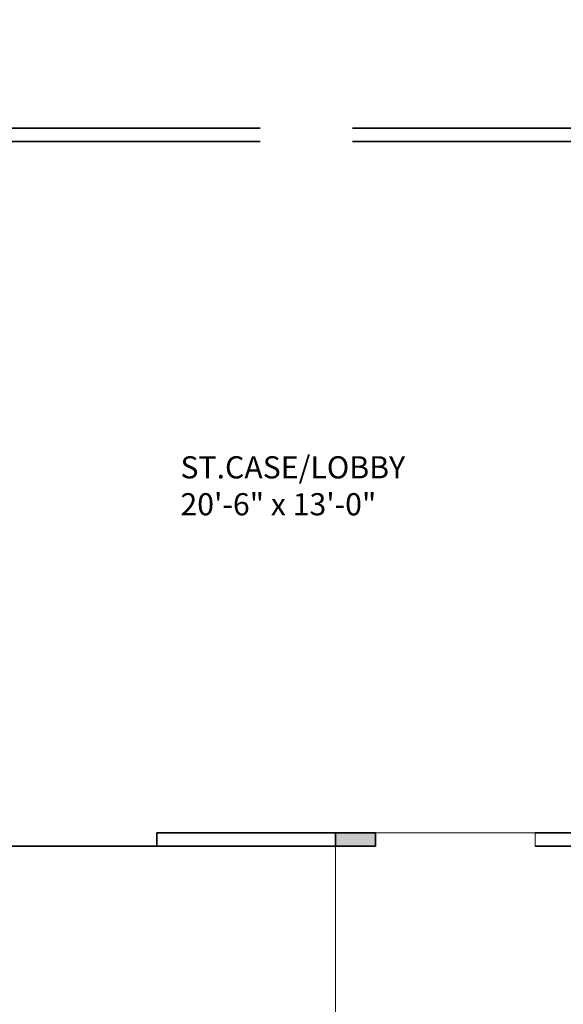
# Model space of a CAD drawing. Units: inches. Extents: x 1002 to 1561, y 1016 to 1994.
# Tile 6 of 8: x 1159 to 1282, y 1283 to 1505. Entities that reach past the tile are written whole.
import ezdxf

# ---------------------------------------------------------------- set-up
doc = ezdxf.new("R2010")
doc.units = ezdxf.units.IN
doc.header["$MEASUREMENT"] = 0
for name, color, linetype, lineweight in [('A-AREA-IDEN', 7, 'Continuous', 18), ('A-WALL', 7, 'Continuous', 35), ('A-WALL-PATT', 7, 'Continuous', 13)]:
    doc.layers.add(name, color=color, linetype=linetype, lineweight=lineweight)
doc.layers.add('A-DOOR', color=30, linetype='Continuous', lineweight=18, true_color=0xf8991e)
doc.styles.get("Standard").update_dxf_attribs({"font": 'arial.ttf'})

msp = doc.modelspace()

# ---------------------------------------------------------------- hatches: boundary and pattern name
at = {"layer": 'A-WALL-PATT'}
h = msp.add_hatch(color=256, dxfattribs=at)
h.dxf.hatch_style = 1
h.paths.add_polyline_path([(1206.434, 1924.784), (1203.434, 1924.784), (1203.434, 1898.155), (1206.434, 1898.155)])
h.paths.add_polyline_path([(1326.434, 1925.745), (1323.434, 1925.745), (1323.434, 1900.458), (1326.434, 1900.458)])
h.paths.add_polyline_path([(1290.434, 1840.51), (1287.434, 1840.51), (1287.434, 1837.51), (1287.434, 1823.284), (1290.434, 1823.284)])
h.paths.add_polyline_path([(1287.434, 1840.51), (1285.684, 1840.51), (1285.684, 1837.51), (1287.434, 1837.51)])
h.paths.add_polyline_path([(1233.434, 1840.51), (1230.434, 1840.51), (1230.434, 1823.284), (1233.434, 1823.284)])
h.paths.add_polyline_path([(1235.119, 1840.51), (1233.434, 1840.51), (1233.434, 1837.51), (1235.119, 1837.51)])
h.paths.add_polyline_path([(1050.434, 1837.51), (1050.434, 1840.51), (1046.434, 1840.51), (1046.434, 1814.619), (1050.434, 1814.619)])
h.paths.add_polyline_path([(1050.434, 1682.088), (1046.434, 1682.088), (1046.434, 1648.51), (1046.434, 1645.51), (1050.434, 1645.51), (1050.434, 1648.51)])
h.paths.add_polyline_path([(1233.434, 1648.51), (1211.636, 1648.51), (1211.636, 1645.51), (1233.434, 1645.51)])
h.paths.add_polyline_path([(1307.549, 1648.51), (1287.434, 1648.51), (1287.434, 1645.51), (1307.549, 1645.51)])
h.paths.add_polyline_path([(1516.434, 1927.595), (1512.434, 1927.595), (1512.434, 1896.846), (1516.434, 1896.846)])
h.paths.add_polyline_path([(1516.434, 1840.51), (1512.434, 1840.51), (1512.434, 1816.31), (1516.434, 1816.31)])
h.paths.add_polyline_path([(1516.434, 1686.827), (1512.434, 1686.827), (1512.434, 1645.51), (1516.434, 1645.51)])
h.paths.add_polyline_path([(1472.434, 1321.51), (1469.434, 1321.51), (1469.434, 1306.51), (1472.434, 1306.51)])
h.paths.add_polyline_path([(1295.733, 1141.51), (1281.793, 1141.51), (1281.793, 1137.51), (1295.733, 1137.51)])
h.paths.add_polyline_path([(1239.434, 1321.51), (1230.434, 1321.51), (1230.434, 1318.51), (1239.434, 1318.51)])
h.paths.add_polyline_path([(1290.434, 1332.122), (1287.434, 1332.122), (1287.434, 1318.51), (1290.434, 1318.51)])
h.paths.add_polyline_path([(1311.434, 1480.51), (1287.434, 1480.51), (1287.434, 1477.51), (1311.434, 1477.51)])
h.paths.add_polyline_path([(1050.434, 1480.51), (1046.434, 1480.51), (1046.434, 1468.51), (1050.434, 1468.51)])
h.paths.add_polyline_path([(1050.434, 1321.51), (1046.434, 1321.51), (1046.434, 1309.51), (1050.434, 1309.51)])
h.paths.add_polyline_path([(1233.434, 1192.382), (1230.434, 1192.382), (1230.434, 1168.702), (1233.434, 1168.702)])
h.paths.add_polyline_path([(1050.434, 1137.51), (1046.434, 1137.51), (1046.434, 1119.51), (1050.434, 1119.51)])
h.paths.add_polyline_path([(1472.434, 1153.51), (1469.434, 1153.51), (1469.434, 1141.51), (1472.434, 1141.51)])
h.paths.add_polyline_path([(1472.434, 1141.51), (1469.434, 1141.51), (1469.434, 1137.51), (1472.434, 1137.51)])

# ---------------------------------------------------------------- linework, layer by layer
at = {"layer": 'A-DOOR'}
for p, q in [((1239.434, 1321.51), (1275.434, 1321.51)), ((1275.434, 1318.51), (1275.434, 1321.51)), ((1230.434, 1277.919), (1230.434, 1318.51))]:
    msp.add_line(p, q, dxfattribs=at)
at = {"layer": 'A-WALL'}
for p, q in [((1156.434, 1480.51), (1213.471, 1480.51)), ((1234.302, 1480.51), (1287.434, 1480.51)), ((1156.434, 1477.51), (1213.471, 1477.51)), ((1234.302, 1477.51), (1287.434, 1477.51)), ((1230.434, 1321.51), (1190.135, 1321.51)), ((1190.135, 1321.51), (1190.135, 1318.51)), ((1230.434, 1321.51), (1239.434, 1321.51)), ((1230.434, 1318.51), (1230.434, 1321.51)), ((1239.434, 1318.51), (1239.434, 1321.51)), ((1275.434, 1321.51), (1287.434, 1321.51)), ((1126.434, 1318.51), (1230.434, 1318.51)), ((1230.434, 1318.51), (1239.434, 1318.51)), ((1275.434, 1318.51), (1413.434, 1318.51))]:
    msp.add_line(p, q, dxfattribs=at)

# ---------------------------------------------------------------- texts
at = {"layer": 'A-AREA-IDEN', "insert": (1195.474, 1406.489), "char_height": 5, "attachment_point": 1}
msp.add_mtext_dynamic_manual_height_columns('ST.CASE/LOBBY\\P20\'-6" x 13\'-0"', width=50.5101, gutter_width=1, heights=[0], dxfattribs=at)

doc.saveas('drawing.dxf')
